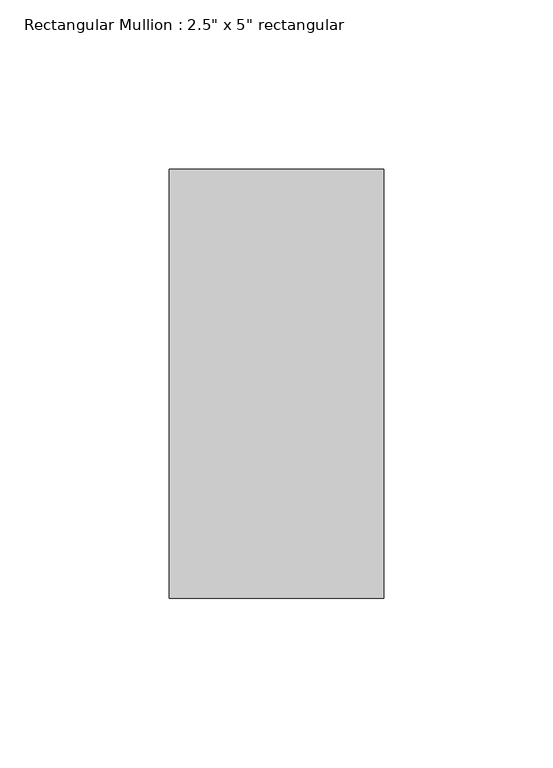
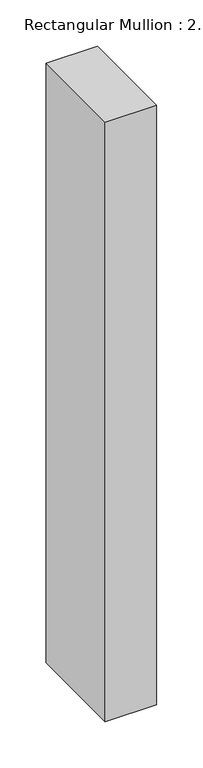
"""IFC4 building model written with IfcOpenShell, lengths in millimetres: member geometry."""

from ifc_helpers import new_model, si_unit, frame, origin, place, context, project, spatial, polyline, outline, extrude, source, transform, mapped, element, save


def member_18a184ad(model_context):
    return source(origin(), model_context, "Body", "SweptSolid", [
        extrude(outline(polyline([(31.75, 63.5), (31.75, -63.5), (-31.75, -63.5), (-31.75, 63.5), (31.75, 63.5)])), frame((0.0, 0.0, -787.4), z_axis=(0.0, 0.0, 1.0), x_axis=(1.0, 0.0, 0.0)), (0.0, 0.0, 1.0), 787.4),
    ])


if __name__ == "__main__":
    model = new_model("IFC4")
    model_context = context("Model", 3, world=origin())
    ifc_project = project(units=[si_unit("LENGTHUNIT", "METRE", prefix="MILLI")], contexts=[model_context])
    site = spatial("IfcSite", under=ifc_project)
    building = spatial("IfcBuilding", under=site)
    placement = place(None, origin())
    member_shape = member_18a184ad(model_context)
    element("IfcMember", 1, ObjectType="Rectangular Mullion : 2.5\" x 5\" rectangular", at=placement, inside=building, context=model_context, shape_type="MappedRepresentation", body=[
        mapped(member_shape, transform((0.0, 0.0, 0.0), x_axis=(1.0, 0.0, 0.0), y_axis=(0.0, 1.0, 0.0), z_axis=(0.0, 0.0, 1.0))),
    ])
    save(model, "model.ifc")

# Revit data of these elements
# Type "Rectangular Mullion : 2.5\" x 5\" rectangular"
#   built-in parameter 1007304 = 0.416667 (stored number, unit not read)
#   built-in parameter 1007301 = 0.104167 (stored number, unit not read)
#   built-in parameter 1007300 = 0.104167 (stored number, unit not read)
